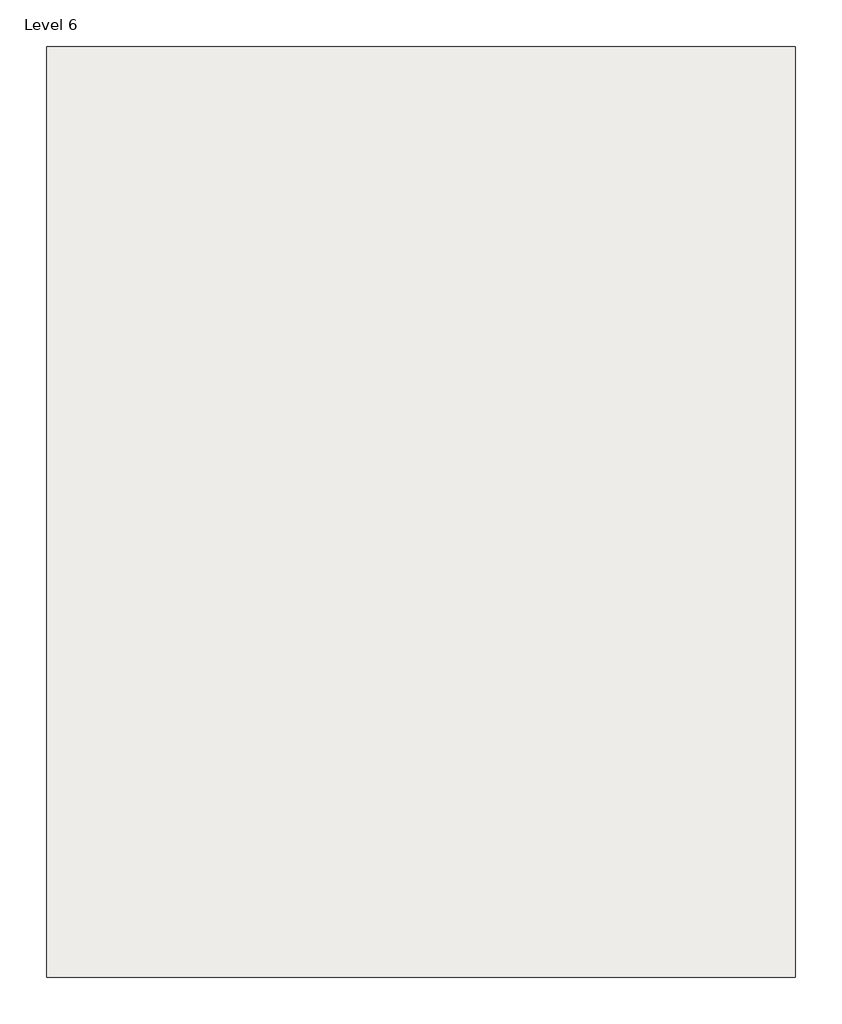
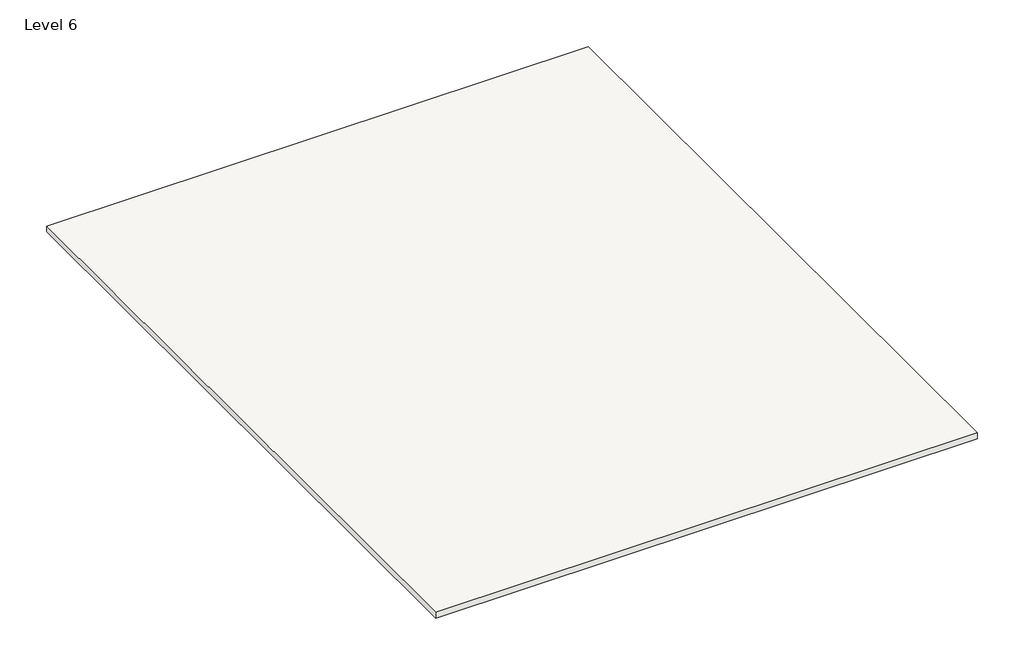
# One storey, incomplete: 1 roof.
"""IFC4 building model written with IfcOpenShell, lengths in millimetres."""

from ifc_helpers import new_model, si_unit, frame, origin, place, context, project, spatial, polyline, outline, extrude, element, save

model = new_model("IFC4")

# Units and contexts
model_context = context("Model", 3, world=origin())
ifc_project = project(units=[si_unit("LENGTHUNIT", "METRE", prefix="MILLI")], contexts=[model_context])

# Site, building, storey
site = spatial("IfcSite", under=ifc_project)
building = spatial("IfcBuilding", under=site)
storey = spatial("IfcBuildingStorey", under=building, Name="Level 6", Elevation=15849.6)

# Roof
placement = place(None, origin())
element("IfcRoof", 1, ObjectType="Generic - 12\"", at=placement, inside=storey, context=model_context, shape_type="SweptSolid", body=[
    extrude(outline(polyline([(-7981.983853, 9646.945119), (5746.716147, 9646.945119), (5746.716147, -7421.854881), (-7981.983853, -7421.854881), (-7981.983853, 9646.945119)])), frame((0.0, 0.0, 15697.2), z_axis=(0.0, 0.0, 1.0), x_axis=(1.0, 0.0, 0.0)), (0.0, 0.0, 1.0), 152.4),
])

save(model, "model.ifc")

# Revit data of these elements
# Type "Generic - 12\""
#   Assembly Code = "B1020"
#   Layers, outside or top first: 0' - 6" no material (function 1)
# Element 1 (IfcRoof, "Generic - 12\"")
#   built-in parameter 1001705 = 52 (stored number, unit not read)
#   built-in parameter 1001701 = -0.5 (stored number, unit not read)
#   built-in parameter 1001710 = 33615
#   Phase Created = New Construction
#   Materials on its faces: "Cherry", "Default Roof", "Wood Planks"
# Materials
#   "Cherry": class "Wood", colour RGB 226 177 128, transparency 0, Description = "Prunus Serotina", Cost = 0
#   "Default Roof": colour RGB 88 101 114, transparency 0, Cost = 0
#   "Wood Planks": class "Wood", colour RGB 193 160 115, transparency 0, Description = "Physical material.", Cost = 0
